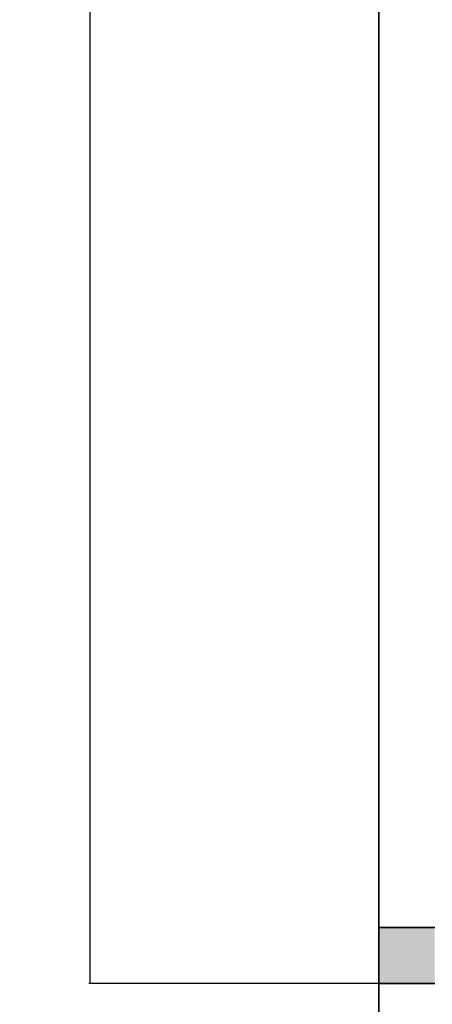
# Model space of a CAD drawing. Units: inches. Extents: x -36302355 to 648, y -221479757 to 75.
# Tile 3 of 37: x 87 to 154, y -583 to -425. Entities that reach past the tile are written whole.
import ezdxf

# ---------------------------------------------------------------- set-up
doc = ezdxf.new("R2010")
doc.units = ezdxf.units.IN
doc.header["$MEASUREMENT"] = 0
for name, color, linetype, lineweight in [('A-ANNO-DIMS', 2, 'Continuous', 18), ('A-COLS', 7, 'Continuous', 35), ('A-COLS-PATT', 242, 'Continuous', 13), ('A-WALL', 7, 'Continuous', 35)]:
    doc.layers.add(name, color=color, linetype=linetype, lineweight=lineweight)
doc.styles.get("Standard").update_dxf_attribs({"font": 'arial.ttf'})
doc.dimstyles.get("Standard").update_dxf_attribs({"dimtxt": 0.18, "dimasz": 0.18, "dimexe": 0.18, "dimexo": 0.0625, "dimgap": 0.09, "dimtad": 0, "dimtih": 1, "dimtoh": 1, "dimdec": 0, "dimzin": 0, "dimdsep": 46, "dimlunit": 3, "dimtxsty": 'Standard', "dimcen": 0.09, "dimadec": 0, "dimazin": 0, "dimtfac": 1, "dimtdec": 0, "dimtofl": 0, "dimtmove": 0, "dimatfit": 3, "dimfxl": 1, "dimtolj": 1, "dimtzin": 0, "dimarcsym": 0})

# ---------------------------------------------------------------- blocks, each defined once
blk = doc.blocks.new('*D7')
at = {"layer": 'A-ANNO-DIMS', "color": 0, "lineweight": -2, "transparency": 16777216}
for p, q in [((145.13, 24.98), (98.63, 24.98)), ((98.81, 24.8), (98.81, -274.37)), ((98.81, -579.84), (98.81, -280.67)), ((145.13, -580.02), (98.63, -580.02))]:
    blk.add_line(p, q, dxfattribs=at)
at = {"layer": 'A-ANNO-DIMS', "color": 0, "transparency": 16777216}
for points in [[(98.78, 24.8), (98.84, 24.8), (98.81, 24.98)], [(98.78, -579.84), (98.84, -579.84), (98.81, -580.02)]]:
    blk.add_solid(points, dxfattribs=at)
at = {"layer": 'Defpoints', "color": 0, "transparency": 16777216}
for p in [(98.81, 24.98), (145.2, 24.98), (145.2, -580.02)]:
    blk.add_point(p, dxfattribs=at)
at = {"layer": 'A-ANNO-DIMS', "color": 0, "transparency": 16777216, "insert": (98.81, -277.52), "char_height": 6, "attachment_point": 5}
blk.add_mtext('\\A1;50\'-5"', dxfattribs=at)

msp = doc.modelspace()

# ---------------------------------------------------------------- hatches: boundary and pattern name
at = {"layer": 'A-COLS-PATT'}
h = msp.add_hatch(color=256, dxfattribs=at)
h.dxf.hatch_style = 1
h.paths.add_polyline_path([(145.2, 24.98), (145.2, 15.98), (154.2, 15.98), (154.2, 24.98)])
h.paths.add_polyline_path([(247.2, 15.98), (247.2, 24.98), (238.2, 24.98), (238.2, 15.98)])
h.paths.add_polyline_path([(387.64, 15.98), (395.7, 15.98), (395.7, 24.98), (387.64, 24.98)])
h.paths.add_polyline_path([(451.26, 24.98), (443.7, 24.98), (443.7, 15.98), (451.26, 15.98)])
h.paths.add_polyline_path([(596.2, 15.98), (605.2, 15.98), (605.2, 24.98), (596.2, 24.98)])
h.paths.add_polyline_path([(238.2, -122.02), (238.2, -131.02), (247.2, -131.02), (247.2, -122.02)])
h.paths.add_polyline_path([(395.7, -122.02), (387.46, -122.02), (387.46, -131.02), (395.7, -131.02)])
h.paths.add_polyline_path([(448.2, -131.02), (453.73, -131.02), (453.73, -122.02), (443.7, -122.02), (443.7, -131.02)])
h.paths.add_polyline_path([(596.2, -131.02), (605.2, -131.02), (605.2, -122.02), (596.2, -122.02)])
h.paths.add_polyline_path([(145.2, -176.97), (154.2, -176.97), (154.2, -167.02), (145.2, -167.02)])
h.paths.add_polyline_path([(314.2, -176.97), (323.2, -176.97), (323.2, -167.02), (314.2, -167.02)])
h.paths.add_polyline_path([(154.2, -314.02), (154.2, -309.52), (145.2, -309.52), (145.2, -314.02)])
h.paths.add_polyline_path([(314.2, -309.52), (314.2, -318.52), (323.2, -318.52), (323.2, -309.52)])
h.paths.add_polyline_path([(448.2, -277.02), (443.7, -277.02), (443.7, -286.02), (448.2, -286.02)])
h.paths.add_polyline_path([(283.2, -370.02), (274.2, -370.02), (274.2, -379.02), (283.2, -379.02), (283.2, -374.52)])
h.paths.add_polyline_path([(154.2, -370.02), (145.2, -370.02), (145.2, -379.02), (154.2, -379.02)])
h.paths.add_polyline_path([(443.2, -374.52), (443.2, -379.02), (452.2, -379.02), (452.2, -374.52)])
h.paths.add_polyline_path([(145.2, -580.02), (154.2, -580.02), (154.2, -571.02), (145.2, -571.02)])
h.paths.add_polyline_path([(274.2, -571.02), (274.2, -580.02), (283.2, -580.02), (283.2, -571.02)])
h.paths.add_polyline_path([(443.2, -580.02), (452.2, -580.02), (452.2, -571.02), (443.2, -571.02)])

# ---------------------------------------------------------------- linework, layer by layer
at = {"layer": 'A-COLS'}
for p, q in [((145.2, -571.02), (154.2, -571.02)), ((145.2, -580.02), (154.2, -580.02))]:
    msp.add_line(p, q, dxfattribs=at)
at = {"layer": 'A-WALL'}
msp.add_line((145.2, -167.02), (145.2, -722.02), dxfattribs=at)

# ---------------------------------------------------------------- dimensions: what is measured, and where the dimension line sits
at = {"layer": 'A-ANNO-DIMS'}
dim = msp.add_linear_dim(base=(98.81, 24.98), p1=(145.2, -580.02), p2=(145.2, 24.98), angle=90, dimstyle='Standard', override={"dimtxt": 6, "dimclrd": 0, "dimclre": 0, "dimclrt": 0}, dxfattribs=at)
dim.commit()
dim.dimension.update_dxf_attribs({"geometry": '*D7', "text_midpoint": (98.81, -277.52)})

doc.saveas('drawing.dxf')
